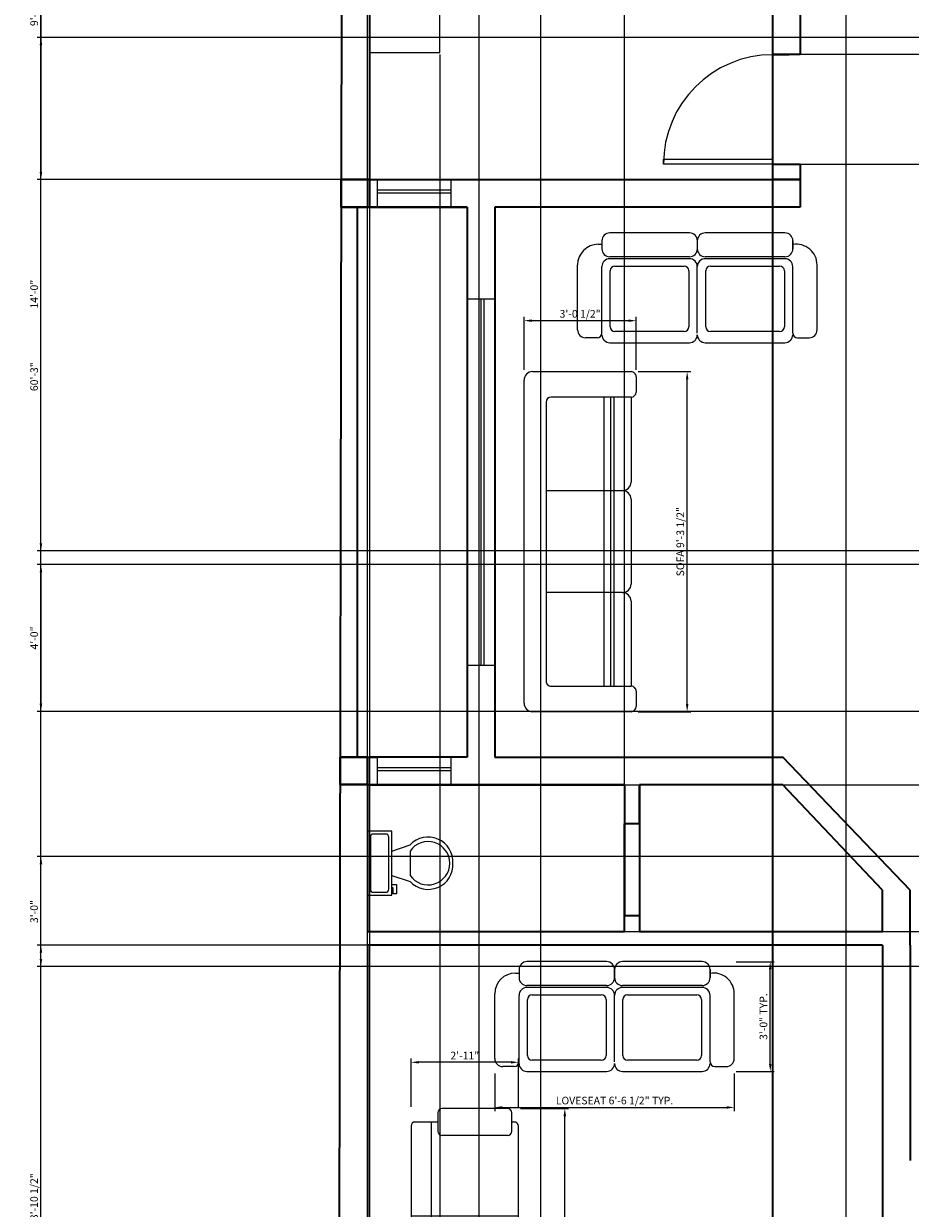
# Model space of a CAD drawing. Units: inches. Extents: x 1624 to 3956, y 1589 to 5028.
# Tile 2 of 16: x 1624 to 1915, y 1862 to 2250. Entities that reach past the tile are written whole.
import ezdxf

# ---------------------------------------------------------------- set-up
doc = ezdxf.new("R2010")
doc.units = ezdxf.units.IN
for name, color, linetype, lineweight in [('A-ANNO-DIMS', 2, 'Continuous', 13), ('A-COLS', 1, 'Continuous', 40), ('A-DOOR', 3, 'Continuous', 18), ('A-FLOR-CASE', 32, 'Continuous', 25), ('A-FLOR-FIXT', 9, 'Continuous', 18), ('A-FURN', 8, 'Continuous', 18), ('A-GLAZ', 4, 'Continuous', 18), ('A-WALL', 7, 'Continuous', 35)]:
    doc.layers.add(name, color=color, linetype=linetype, lineweight=lineweight)
doc.styles.get("Standard").update_dxf_attribs({"font": 'arial.ttf'})
doc.dimstyles.new('Copy of ISO-25', dxfattribs={"dimtxt": 2.5, "dimasz": 2.5, "dimexe": 1.25, "dimexo": 0.625, "dimtad": 1, "dimdec": 1, "dimlunit": 4, "dimtxsty": 'Standard', "dimcen": 2.5, "dimadec": 0, "dimazin": 0, "dimtfac": 1, "dimtdec": 1, "dimtmove": 0, "dimatfit": 3, "dimfxl": 1, "dimarcsym": 0})

# ---------------------------------------------------------------- blocks, each defined once
blk = doc.blocks.new('*U6')
for p, q in [((0, 0), (0, -6)), ((40, 0), (40, -6))]:
    blk.add_line(p, q)
blk.add_lwpolyline([(0, 0), (0, 40), (1.75, 40), (1.75, 0)], close=True)
blk.add_arc((0, 0), 40, 0, 90)
blk = doc.blocks.new('A$C05BA3A2B')
for p, q in [((0.05, 0.6596), (1.95, 0.6596)), ((0.05, 0.6596), (1.95, 0.6596)), ((0.05, 0.6596), (1.95, 0.6596)), ((0, 0.03), (0, 0.6096)), ((0, 0.03), (0, 0.6096)), ((0, 0.03), (0, 0.6096)), ((2, 0.6096), (2, 0.03)), ((2, 0.6096), (2, 0.03)), ((2, 0.6096), (2, 0.03)), ((0.15, 0.5), (0.15, 0.03)), ((0.15, 0.5), (0.15, 0.03)), ((0.15, 0.5), (0.15, 0.03)), ((1.82, 0.53), (0.18, 0.53)), ((1.82, 0.53), (0.18, 0.53)), ((1.82, 0.53), (0.18, 0.53)), ((0.7, 0.08), (0.7, 0.53)), ((0.7, 0.08), (0.7, 0.53)), ((0.7, 0.08), (0.7, 0.53)), ((1.3, 0.53), (1.3, 0.08)), ((1.3, 0.53), (1.3, 0.08)), ((1.3, 0.53), (1.3, 0.08)), ((1.85, 0.03), (1.85, 0.5)), ((1.85, 0.03), (1.85, 0.5)), ((1.85, 0.03), (1.85, 0.5)), ((1.85, 0.1908), (0.15, 0.1908)), ((1.85, 0.1908), (0.15, 0.1908)), ((1.85, 0.1908), (0.15, 0.1908)), ((1.85, 0.1508), (0.15, 0.1508)), ((1.85, 0.1508), (0.15, 0.1508)), ((1.85, 0.1508), (0.15, 0.1508)), ((1.85, 0.1308), (0.15, 0.1308)), ((1.85, 0.1308), (0.15, 0.1308)), ((1.85, 0.1308), (0.15, 0.1308)), ((0.12, 0), (0.03, 0)), ((0.12, 0), (0.03, 0)), ((0.12, 0), (0.03, 0)), ((0.65, 0.03), (0.15, 0.03)), ((0.65, 0.03), (0.15, 0.03)), ((0.65, 0.03), (0.15, 0.03)), ((1.25, 0.03), (0.75, 0.03)), ((1.25, 0.03), (0.75, 0.03)), ((1.25, 0.03), (0.75, 0.03)), ((1.85, 0.03), (1.35, 0.03)), ((1.85, 0.03), (1.35, 0.03)), ((1.85, 0.03), (1.35, 0.03)), ((1.97, 0), (1.88, 0)), ((1.97, 0), (1.88, 0)), ((1.97, 0), (1.88, 0))]:
    blk.add_line(p, q)
for centre, radius, start, end in [((0.05, 0.6096), 0.05, 90, 180), ((0.05, 0.6096), 0.05, 90, 180), ((0.05, 0.6096), 0.05, 90, 180), ((1.95, 0.6096), 0.05, 0, 90), ((1.95, 0.6096), 0.05, 0, 90), ((1.95, 0.6096), 0.05, 0, 90), ((0.18, 0.5), 0.03, 90, 180), ((0.18, 0.5), 0.03, 90, 180), ((0.18, 0.5), 0.03, 90, 180), ((1.82, 0.5), 0.03, 0, 90), ((1.82, 0.5), 0.03, 0, 90), ((1.82, 0.5), 0.03, 0, 90), ((0.65, 0.08), 0.05, 270, 0), ((0.65, 0.08), 0.05, 270, 0), ((0.65, 0.08), 0.05, 270, 0), ((0.75, 0.08), 0.05, 180, 270), ((0.75, 0.08), 0.05, 180, 270), ((0.75, 0.08), 0.05, 180, 270), ((1.25, 0.08), 0.05, 270, 0), ((1.25, 0.08), 0.05, 270, 0), ((1.25, 0.08), 0.05, 270, 0), ((1.35, 0.08), 0.05, 180, 270), ((1.35, 0.08), 0.05, 180, 270), ((1.35, 0.08), 0.05, 180, 270), ((0.03, 0.03), 0.03, 180, 270), ((0.03, 0.03), 0.03, 180, 270), ((0.03, 0.03), 0.03, 180, 270), ((0.12, 0.03), 0.03, 270, 0), ((0.12, 0.03), 0.03, 270, 0), ((0.12, 0.03), 0.03, 270, 0), ((1.88, 0.03), 0.03, 180, 270), ((1.88, 0.03), 0.03, 180, 270), ((1.88, 0.03), 0.03, 180, 270), ((1.97, 0.03), 0.03, 270, 0), ((1.97, 0.03), 0.03, 270, 0), ((1.97, 0.03), 0.03, 270, 0)]:
    blk.add_arc(centre, radius, start, end)
blk = doc.blocks.new('*U14')
for p, q in [((241.3, -152.4), (241.3, -50.8)), ((-254, -215.9), (-203.2, -215.9)), ((-254, -241.3), (-254, -215.9)), ((-177.8, -241.3), (-254, -241.3)), ((-203.2, -215.9), (-203.2, -203.2)), ((-177.8, -203.2), (-177.8, -241.3)), ((-101.6, -203.2), (-152.4, -355.6)), ((101.6, -203.2), (152.4, -355.6)), ((101.6, -355.6), (-101.6, -355.6))]:
    blk.add_line(p, q)
blk.add_lwpolyline([(266.7, -203.2), (266.7, 0), (-266.7, 0), (-266.7, -203.2)], close=True)
for points in [[(-241.3, -50.8), (-241.3, -152.4)], [(215.9, -25.4), (-215.9, -25.4)], [(-215.9, -177.8), (215.9, -177.8)]]:
    blk.add_lwpolyline(points)
for centre, radius, start, end in [((-219.075, -47.625), 22.45064, 81.8699, 188.1301), ((219.075, -47.625), 22.45064, 351.8699, 98.1301), ((-219.075, -155.575), 22.45064, 171.869898, 278.1301), ((219.075, -155.575), 22.45064, 261.8699, 8.1301), ((-12.12088, -505.93752), 205.61935, 133.01722, 273.38), ((0.94996, -504.77674), 181.02486, 124.50543, 269.7), ((-0.94742, -504.77674), 181.02486, 270.3, 55.4946), ((12.12342, -505.93752), 205.61935, 266.62, 46.9828)]:
    blk.add_arc(centre, radius, start, end)
blk = doc.blocks.new('A$C555E41E5')
for p, q in [((0.13, 0.8), (0.8, 0.8)), ((0.8, 0.8), (0.8, 0)), ((0.8, 0.8), (0.8, 0)), ((1.5, 0.8), (0.8, 0.8)), ((2.17, 0.8), (1.5, 0.8)), ((1.5, 0.8), (1.5, 0)), ((1.5, 0.8), (1.5, 0)), ((0.1, 0.6), (0.1, 0.77)), ((2.2, 0.6), (2.2, 0.77)), ((0.1, 0.65), (0.8, 0.65)), ((1.53, 0.65), (0.8, 0.65)), ((2.2, 0.65), (1.5, 0.65)), ((0, 0.08), (0, 0.57)), ((0.03, 0.6), (0.17, 0.6)), ((0.2, 0.08), (0.2, 0.57)), ((2.1, 0.08), (2.1, 0.57)), ((2.27, 0.6), (2.13, 0.6)), ((2.3, 0.08), (2.3, 0.57)), ((0.17, 0.05), (0.03, 0.05)), ((0.1, 0.03), (0.1, 0.05)), ((0.8, 0), (0.13, 0)), ((0.8, 0), (1.5, 0)), ((1.5, 0), (2.17, 0)), ((2.13, 0.05), (2.27, 0.05)), ((2.2, 0.03), (2.2, 0.05))]:
    blk.add_line(p, q)
for centre, start, end in [((0.13, 0.77), 90, 180), ((2.17, 0.77), 0, 90), ((0.03, 0.57), 90, 180), ((0.17, 0.57), 0, 90), ((2.13, 0.57), 90, 180), ((2.27, 0.57), 0, 90), ((0.03, 0.08), 180, 270), ((0.13, 0.03), 180, 270), ((0.17, 0.08), 270, 0), ((2.13, 0.08), 180, 270), ((2.17, 0.03), 270, 0), ((2.27, 0.08), 270, 0)]:
    blk.add_arc(centre, 0.03, start, end)
blk = doc.blocks.new('A$C2BCD7A6E')
blk.add_blockref('A$C555E41E5', (0, 0))
blk = doc.blocks.new('A$C243830B6')
for p, q in [((0.7024, 0.6896), (0.2024, 0.6896)), ((1.3021, 0.6896), (0.8021, 0.6896)), ((0.13, 0.618), (0.15, 0.618)), ((0.1524, 0.6396), (0.1524, 0.5896)), ((0.7521, 0.6396), (0.7521, 0.5896)), ((0.7524, 0.5896), (0.7524, 0.6396)), ((1.3521, 0.6396), (1.3521, 0.5896)), ((1.3524, 0.5896), (1.3524, 0.6396)), ((0.7024, 0.5396), (0.2024, 0.5396)), ((0.7021, 0.5276), (0.2024, 0.5276)), ((1.3021, 0.5396), (0.8021, 0.5396)), ((1.3018, 0.5276), (0.8021, 0.5276)), ((0, 0.0808), (0, 0.488)), ((0.1524, 0.0608), (0.1524, 0.4776)), ((0.2048, 0.1005), (0.2048, 0.4515)), ((0.2348, 0.4815), (0.6691, 0.4815)), ((0.6991, 0.4515), (0.6991, 0.1005)), ((0.7521, 0.0608), (0.7521, 0.4776)), ((0.7521, 0.0608), (0.7521, 0.4776)), ((0.8045, 0.1005), (0.8045, 0.4515)), ((0.8345, 0.4815), (1.2688, 0.4815)), ((1.2988, 0.4515), (1.2988, 0.1005)), ((1.3518, 0.0608), (1.3518, 0.4776)), ((1.3521, 0.0608), (1.3521, 0.4776)), ((1.3521, 0.0608), (1.3521, 0.4776)), ((1.5043, 0.0808), (1.5043, 0.488)), ((0.1224, 0.0308), (0.05, 0.0308)), ((0.2024, 0), (0.7021, 0)), ((0.6691, 0.0705), (0.2348, 0.0705)), ((0.8021, 0), (1.3018, 0)), ((1.2688, 0.0705), (0.8345, 0.0705)), ((1.382, 0.0308), (1.4543, 0.0308))]:
    blk.add_line(p, q)
for centre, radius, start, end in [((0.2024, 0.6396), 0.05, 90, 180), ((0.7024, 0.6396), 0.05, 0, 90), ((0.8021, 0.6396), 0.05, 90, 180), ((1.3021, 0.6396), 0.05, 0, 90), ((0.13, 0.488), 0.13, 90, 180), ((1.3743, 0.488), 0.13, 0, 99.86144), ((0.2024, 0.5896), 0.05, 180, 270), ((0.2024, 0.4776), 0.05, 90, 180), ((0.7021, 0.4776), 0.05, 0, 90), ((0.7024, 0.5896), 0.05, 270, 0), ((0.8021, 0.5896), 0.05, 180, 270), ((0.8021, 0.4776), 0.05, 90, 180), ((1.3018, 0.4776), 0.05, 0, 90), ((1.3021, 0.5896), 0.05, 270, 0), ((0.2348, 0.4515), 0.03, 90, 180), ((0.6691, 0.4515), 0.03, 0, 90), ((0.8345, 0.4515), 0.03, 90, 180), ((1.2688, 0.4515), 0.03, 0, 90), ((0.05, 0.0808), 0.05, 180, 270), ((0.2348, 0.1005), 0.03, 180, 270), ((0.6691, 0.1005), 0.03, 270, 0), ((0.8345, 0.1005), 0.03, 180, 270), ((1.2688, 0.1005), 0.03, 270, 0), ((1.4543, 0.0808), 0.05, 270, 0), ((0.1224, 0.0608), 0.03, 270, 0), ((0.2024, 0.05), 0.05, 180, 270), ((0.7021, 0.05), 0.05, 270, 0), ((0.8021, 0.05), 0.05, 180, 270), ((1.3018, 0.05), 0.05, 270, 0), ((1.382, 0.0608), 0.03, 180, 270)]:
    blk.add_arc(centre, radius, start, end)
blk = doc.blocks.new('WINDOW-24IN')
for p, q in [((0, 0), (0, 9)), ((24, 9), (24, 0)), ((24, 5.5), (0, 5.5)), ((24, 4.5), (0, 4.5))]:
    blk.add_line(p, q)
blk = doc.blocks.new('*D56')
at = {"layer": 'A-ANNO-DIMS', "color": 0, "lineweight": -2, "transparency": 16777216}
for p, q in [((1778.6, 1906.33), (1778.6, 1893.95)), ((1856.98, 1906.33), (1856.98, 1893.95)), ((1781.1, 1895.2), (1854.48, 1895.2))]:
    blk.add_line(p, q, dxfattribs=at)
at = {"layer": 'A-ANNO-DIMS', "color": 0, "transparency": 16777216}
for points in [[(1781.1, 1895.61), (1781.1, 1894.78), (1778.6, 1895.2)], [(1854.48, 1895.61), (1854.48, 1894.78), (1856.98, 1895.2)]]:
    blk.add_solid(points, dxfattribs=at)
at = {"layer": 'Defpoints', "color": 0, "transparency": 16777216}
for p in [(1778.6, 1906.96), (1856.98, 1906.96), (1856.98, 1895.2)]:
    blk.add_point(p, dxfattribs=at)
at = {"layer": 'A-ANNO-DIMS', "color": 0, "transparency": 16777216, "insert": (1817.79, 1897.12), "char_height": 2.5, "attachment_point": 5}
blk.add_mtext('LOVESEAT 6\'-6 1/2" TYP.', dxfattribs=at)
blk = doc.blocks.new('*D57')
at = {"layer": 'A-ANNO-DIMS', "color": 0, "lineweight": -2, "transparency": 16777216}
for p, q in [((1857.61, 1942.89), (1869.99, 1942.89)), ((1868.74, 1909.46), (1868.74, 1940.39)), ((1857.61, 1906.96), (1869.99, 1906.96))]:
    blk.add_line(p, q, dxfattribs=at)
at = {"layer": 'A-ANNO-DIMS', "color": 0, "transparency": 16777216}
for points in [[(1868.32, 1940.39), (1869.16, 1940.39), (1868.74, 1942.89)], [(1868.32, 1909.46), (1869.16, 1909.46), (1868.74, 1906.96)]]:
    blk.add_solid(points, dxfattribs=at)
at = {"layer": 'Defpoints', "color": 0, "transparency": 16777216}
for p in [(1856.98, 1942.89), (1868.74, 1942.89), (1856.98, 1906.96)]:
    blk.add_point(p, dxfattribs=at)
at = {"layer": 'A-ANNO-DIMS', "color": 0, "transparency": 16777216, "insert": (1866.84, 1924.92), "char_height": 2.5, "attachment_point": 5, "rotation": 90}
blk.add_mtext('3\'-0" TYP.', dxfattribs=at)
blk = doc.blocks.new('*D62')
at = {"layer": 'A-ANNO-DIMS', "color": 0, "lineweight": -2, "transparency": 16777216}
for p, q in [((1825.5, 2135.94), (1842.81, 2135.94)), ((1841.56, 2027.19), (1841.56, 2133.44)), ((1825.5, 2024.69), (1842.81, 2024.69))]:
    blk.add_line(p, q, dxfattribs=at)
at = {"layer": 'A-ANNO-DIMS', "color": 0, "transparency": 16777216}
for points in [[(1841.14, 2133.44), (1841.98, 2133.44), (1841.56, 2135.94)], [(1841.14, 2027.19), (1841.98, 2027.19), (1841.56, 2024.69)]]:
    blk.add_solid(points, dxfattribs=at)
at = {"layer": 'Defpoints', "color": 0, "transparency": 16777216}
for p in [(1824.87, 2135.94), (1841.56, 2135.94), (1824.87, 2024.69)]:
    blk.add_point(p, dxfattribs=at)
at = {"layer": 'A-ANNO-DIMS', "color": 0, "transparency": 16777216, "insert": (1839.64, 2080.31), "char_height": 2.5, "attachment_point": 5, "rotation": 90}
blk.add_mtext('SOFA 9\'-3 1/2"', dxfattribs=at)
blk = doc.blocks.new('*D63')
at = {"layer": 'A-ANNO-DIMS', "color": 0, "lineweight": -2, "transparency": 16777216}
for p, q in [((1788.18, 2136.56), (1788.18, 2153.87)), ((1822.37, 2152.62), (1790.68, 2152.62)), ((1824.87, 2136.56), (1824.87, 2153.87))]:
    blk.add_line(p, q, dxfattribs=at)
at = {"layer": 'A-ANNO-DIMS', "color": 0, "transparency": 16777216}
for points in [[(1790.68, 2153.04), (1790.68, 2152.21), (1788.18, 2152.62)], [(1822.37, 2153.04), (1822.37, 2152.21), (1824.87, 2152.62)]]:
    blk.add_solid(points, dxfattribs=at)
at = {"layer": 'Defpoints', "color": 0, "transparency": 16777216}
for p in [(1788.18, 2152.62), (1788.18, 2135.94), (1824.87, 2135.94)]:
    blk.add_point(p, dxfattribs=at)
at = {"layer": 'A-ANNO-DIMS', "color": 0, "transparency": 16777216, "insert": (1806.53, 2154.54), "char_height": 2.5, "attachment_point": 5}
blk.add_mtext('3\'-0 1/2"', dxfattribs=at)
blk = doc.blocks.new('*D64')
at = {"layer": 'A-ANNO-DIMS', "color": 0, "lineweight": -2, "transparency": 16777216}
for p, q in [((1787, 1894.81), (1802.77, 1894.81)), ((1801.52, 1796.3), (1801.52, 1892.31)), ((1787, 1793.8), (1802.77, 1793.8))]:
    blk.add_line(p, q, dxfattribs=at)
at = {"layer": 'A-ANNO-DIMS', "color": 0, "transparency": 16777216}
for points in [[(1801.11, 1892.31), (1801.94, 1892.31), (1801.52, 1894.81)], [(1801.11, 1796.3), (1801.94, 1796.3), (1801.52, 1793.8)]]:
    blk.add_solid(points, dxfattribs=at)
at = {"layer": 'Defpoints', "color": 0, "transparency": 16777216}
for p in [(1786.37, 1894.81), (1801.52, 1894.81), (1786.37, 1793.8)]:
    blk.add_point(p, dxfattribs=at)
at = {"layer": 'A-ANNO-DIMS', "color": 0, "transparency": 16777216, "insert": (1799.6, 1844.31), "char_height": 2.5, "attachment_point": 5, "rotation": 90}
blk.add_mtext('SOFA 8\'-5"', dxfattribs=at)
blk = doc.blocks.new('*D65')
at = {"layer": 'A-ANNO-DIMS', "color": 0, "lineweight": -2, "transparency": 16777216}
for p, q in [((1751.23, 1895.44), (1751.23, 1911.22)), ((1786.37, 1895.44), (1786.37, 1911.22)), ((1783.87, 1909.97), (1753.73, 1909.97))]:
    blk.add_line(p, q, dxfattribs=at)
at = {"layer": 'A-ANNO-DIMS', "color": 0, "transparency": 16777216}
for points in [[(1753.73, 1910.38), (1753.73, 1909.55), (1751.23, 1909.97)], [(1783.87, 1910.38), (1783.87, 1909.55), (1786.37, 1909.97)]]:
    blk.add_solid(points, dxfattribs=at)
at = {"layer": 'Defpoints', "color": 0, "transparency": 16777216}
for p in [(1751.23, 1909.97), (1751.23, 1894.81), (1786.37, 1894.81)]:
    blk.add_point(p, dxfattribs=at)
at = {"layer": 'A-ANNO-DIMS', "color": 0, "transparency": 16777216, "insert": (1768.8, 1911.85), "char_height": 2.5, "attachment_point": 5}
blk.add_mtext('2\'-11"', dxfattribs=at)
blk = doc.blocks.new('*D69')
at = {"layer": 'A-ANNO-DIMS', "color": 0, "lineweight": -2, "transparency": 16777216}
for p, q in [((1727.95, 2495.79), (1628.86, 2495.79)), ((1630.11, 1775.29), (1630.11, 2493.29)), ((1726.95, 1772.79), (1628.86, 1772.79))]:
    blk.add_line(p, q, dxfattribs=at)
at = {"layer": 'A-ANNO-DIMS', "color": 0, "transparency": 16777216}
for points in [[(1629.69, 2493.29), (1630.53, 2493.29), (1630.11, 2495.79)], [(1629.69, 1775.29), (1630.53, 1775.29), (1630.11, 1772.79)]]:
    blk.add_solid(points, dxfattribs=at)
at = {"layer": 'Defpoints', "color": 0, "transparency": 16777216}
for p in [(1630.11, 2495.79), (1728.58, 2495.79), (1727.58, 1772.79)]:
    blk.add_point(p, dxfattribs=at)
at = {"layer": 'A-ANNO-DIMS', "color": 0, "transparency": 16777216, "insert": (1628.21, 2134.29), "char_height": 2.5, "attachment_point": 5, "rotation": 90}
blk.add_mtext('60\'-3"', dxfattribs=at)
blk = doc.blocks.new('*D75')
at = {"layer": 'A-ANNO-DIMS', "color": 0, "lineweight": -2, "transparency": 16777216}
for p, q in [((1737.58, 2486.17), (1737.58, 1589.9)), ((1793.58, 2486.17), (1793.58, 1589.9)), ((1740.08, 1591.15), (1791.08, 1591.15))]:
    blk.add_line(p, q, dxfattribs=at)
at = {"layer": 'A-ANNO-DIMS', "color": 0, "transparency": 16777216}
for points in [[(1740.08, 1591.57), (1740.08, 1590.73), (1737.58, 1591.15)], [(1791.08, 1591.57), (1791.08, 1590.73), (1793.58, 1591.15)]]:
    blk.add_solid(points, dxfattribs=at)
at = {"layer": 'Defpoints', "color": 0, "transparency": 16777216}
for p in [(1737.58, 2486.79), (1793.58, 2486.79), (1793.58, 1591.15)]:
    blk.add_point(p, dxfattribs=at)
at = {"layer": 'A-ANNO-DIMS', "color": 0, "transparency": 16777216, "insert": (1765.58, 1593.05), "char_height": 2.5, "attachment_point": 5}
blk.add_mtext('4\'-8"', dxfattribs=at)
blk = doc.blocks.new('*D82')
at = {"layer": 'A-ANNO-DIMS', "color": 0, "lineweight": -2, "transparency": 16777216}
for p, q in [((1737.58, 2306.17), (1737.58, 1589.9)), ((1869.56, 2306.17), (1869.56, 1589.9)), ((1740.08, 1591.15), (1867.06, 1591.15))]:
    blk.add_line(p, q, dxfattribs=at)
at = {"layer": 'A-ANNO-DIMS', "color": 0, "transparency": 16777216}
for points in [[(1740.08, 1591.57), (1740.08, 1590.73), (1737.58, 1591.15)], [(1867.06, 1591.57), (1867.06, 1590.73), (1869.56, 1591.15)]]:
    blk.add_solid(points, dxfattribs=at)
at = {"layer": 'Defpoints', "color": 0, "transparency": 16777216}
for p in [(1737.58, 2306.79), (1869.56, 2306.79), (1869.56, 1591.15)]:
    blk.add_point(p, dxfattribs=at)
at = {"layer": 'A-ANNO-DIMS', "color": 0, "transparency": 16777216, "insert": (1803.57, 1593.05), "char_height": 2.5, "attachment_point": 5}
blk.add_mtext('11\'-0"', dxfattribs=at)
blk = doc.blocks.new('*D83')
at = {"layer": 'A-ANNO-DIMS', "color": 0, "lineweight": -2, "transparency": 16777216}
for p, q in [((1868.93, 2306.79), (1628.86, 2306.79)), ((1630.11, 2304.29), (1630.11, 2201.29)), ((1868.93, 2198.79), (1628.86, 2198.79))]:
    blk.add_line(p, q, dxfattribs=at)
at = {"layer": 'A-ANNO-DIMS', "color": 0, "transparency": 16777216}
for points in [[(1629.69, 2304.29), (1630.53, 2304.29), (1630.11, 2306.79)], [(1629.69, 2201.29), (1630.53, 2201.29), (1630.11, 2198.79)]]:
    blk.add_solid(points, dxfattribs=at)
at = {"layer": 'Defpoints', "color": 0, "transparency": 16777216}
for p in [(1869.56, 2306.79), (1630.11, 2198.79), (1869.56, 2198.79)]:
    blk.add_point(p, dxfattribs=at)
at = {"layer": 'A-ANNO-DIMS', "color": 0, "transparency": 16777216, "insert": (1628.21, 2252.79), "char_height": 2.5, "attachment_point": 5, "rotation": 90}
blk.add_mtext('9\'-0"', dxfattribs=at)
blk = doc.blocks.new('*D84')
at = {"layer": 'A-ANNO-DIMS', "color": 0, "lineweight": -2, "transparency": 16777216}
for p, q in [((1904.9, 1948.29), (1628.86, 1948.29)), ((1630.11, 1784.29), (1630.11, 1945.79)), ((1904.9, 1781.79), (1628.86, 1781.79))]:
    blk.add_line(p, q, dxfattribs=at)
at = {"layer": 'A-ANNO-DIMS', "color": 0, "transparency": 16777216}
for points in [[(1629.69, 1945.79), (1630.53, 1945.79), (1630.11, 1948.29)], [(1629.69, 1784.29), (1630.53, 1784.29), (1630.11, 1781.79)]]:
    blk.add_solid(points, dxfattribs=at)
at = {"layer": 'Defpoints', "color": 0, "transparency": 16777216}
for p in [(1630.11, 1948.29), (1905.53, 1948.29), (1905.53, 1781.79)]:
    blk.add_point(p, dxfattribs=at)
at = {"layer": 'A-ANNO-DIMS', "color": 0, "transparency": 16777216, "insert": (1628.19, 1865.04), "char_height": 2.5, "attachment_point": 5, "rotation": 90}
blk.add_mtext('13\'-10 1/2"', dxfattribs=at)
blk = doc.blocks.new('*D86')
at = {"layer": 'A-ANNO-DIMS', "color": 0, "lineweight": -2, "transparency": 16777216}
for p, q in [((1737.01, 1953.42), (1737.01, 2612.84)), ((1821.01, 1953.42), (1821.01, 2612.84)), ((1739.51, 2611.59), (1818.51, 2611.59))]:
    blk.add_line(p, q, dxfattribs=at)
at = {"layer": 'A-ANNO-DIMS', "color": 0, "transparency": 16777216}
for points in [[(1739.51, 2612.01), (1739.51, 2611.18), (1737.01, 2611.59)], [(1818.51, 2612.01), (1818.51, 2611.18), (1821.01, 2611.59)]]:
    blk.add_solid(points, dxfattribs=at)
at = {"layer": 'Defpoints', "color": 0, "transparency": 16777216}
for p in [(1821.01, 2611.59), (1737.01, 1952.79), (1821.01, 1952.79)]:
    blk.add_point(p, dxfattribs=at)
at = {"layer": 'A-ANNO-DIMS', "color": 0, "transparency": 16777216, "insert": (1779.01, 2613.5), "char_height": 2.5, "attachment_point": 5}
blk.add_mtext('7\'-0"', dxfattribs=at)
blk = doc.blocks.new('*D87')
at = {"layer": 'A-ANNO-DIMS', "color": 0, "lineweight": -2, "transparency": 16777216}
for p, q in [((1737.64, 2000.79), (2217.63, 2000.79)), ((2216.38, 1998.29), (2216.38, 1955.29)), ((1737.64, 1952.79), (2217.63, 1952.79))]:
    blk.add_line(p, q, dxfattribs=at)
at = {"layer": 'A-ANNO-DIMS', "color": 0, "transparency": 16777216}
for points in [[(2215.96, 1998.29), (2216.8, 1998.29), (2216.38, 2000.79)], [(2215.96, 1955.29), (2216.8, 1955.29), (2216.38, 1952.79)]]:
    blk.add_solid(points, dxfattribs=at)
at = {"layer": 'Defpoints', "color": 0, "transparency": 16777216}
for p in [(1737.01, 2000.79), (1737.01, 1952.79), (2216.38, 1952.79)]:
    blk.add_point(p, dxfattribs=at)
at = {"layer": 'A-ANNO-DIMS', "color": 0, "transparency": 16777216, "insert": (2214.48, 1976.79), "char_height": 2.5, "attachment_point": 5, "rotation": 90}
blk.add_mtext('4\'-0"', dxfattribs=at)
blk = doc.blocks.new('*D91')
at = {"layer": 'A-ANNO-DIMS', "color": 0, "lineweight": -2, "transparency": 16777216}
for p, q in [((2054.95, 1977.29), (1628.86, 1977.29)), ((1630.11, 1943.79), (1630.11, 1974.79)), ((2054.95, 1941.29), (1628.86, 1941.29))]:
    blk.add_line(p, q, dxfattribs=at)
at = {"layer": 'A-ANNO-DIMS', "color": 0, "transparency": 16777216}
for points in [[(1629.69, 1974.79), (1630.53, 1974.79), (1630.11, 1977.29)], [(1629.69, 1943.79), (1630.53, 1943.79), (1630.11, 1941.29)]]:
    blk.add_solid(points, dxfattribs=at)
at = {"layer": 'Defpoints', "color": 0, "transparency": 16777216}
for p in [(1630.11, 1977.29), (2055.58, 1977.29), (2055.58, 1941.29)]:
    blk.add_point(p, dxfattribs=at)
at = {"layer": 'A-ANNO-DIMS', "color": 0, "transparency": 16777216, "insert": (1628.21, 1959.29), "char_height": 2.5, "attachment_point": 5, "rotation": 90}
blk.add_mtext('3\'-0"', dxfattribs=at)
blk = doc.blocks.new('*D93')
at = {"layer": 'A-ANNO-DIMS', "color": 0, "lineweight": -2, "transparency": 16777216}
for p, q in [((2090.95, 2072.79), (1628.86, 2072.79)), ((1630.11, 2070.29), (1630.11, 2027.29)), ((2090.95, 2024.79), (1628.86, 2024.79))]:
    blk.add_line(p, q, dxfattribs=at)
at = {"layer": 'A-ANNO-DIMS', "color": 0, "transparency": 16777216}
for points in [[(1629.69, 2070.29), (1630.53, 2070.29), (1630.11, 2072.79)], [(1629.69, 2027.29), (1630.53, 2027.29), (1630.11, 2024.79)]]:
    blk.add_solid(points, dxfattribs=at)
at = {"layer": 'Defpoints', "color": 0, "transparency": 16777216}
for p in [(2091.58, 2072.79), (1630.11, 2024.79), (2091.58, 2024.79)]:
    blk.add_point(p, dxfattribs=at)
at = {"layer": 'A-ANNO-DIMS', "color": 0, "transparency": 16777216, "insert": (1628.21, 2048.79), "char_height": 2.5, "attachment_point": 5, "rotation": 90}
blk.add_mtext('4\'-0"', dxfattribs=at)
blk = doc.blocks.new('*D94')
at = {"layer": 'A-ANNO-DIMS', "color": 0, "lineweight": -2, "transparency": 16777216}
for p, q in [((1893.52, 2315.17), (1893.52, 1589.9)), ((1929.52, 2315.17), (1929.52, 1589.9)), ((1896.02, 1591.15), (1927.02, 1591.15))]:
    blk.add_line(p, q, dxfattribs=at)
at = {"layer": 'A-ANNO-DIMS', "color": 0, "transparency": 16777216}
for points in [[(1896.02, 1591.57), (1896.02, 1590.73), (1893.52, 1591.15)], [(1927.02, 1591.57), (1927.02, 1590.73), (1929.52, 1591.15)]]:
    blk.add_solid(points, dxfattribs=at)
at = {"layer": 'Defpoints', "color": 0, "transparency": 16777216}
for p in [(1893.52, 2315.79), (1929.52, 2315.79), (1929.52, 1591.15)]:
    blk.add_point(p, dxfattribs=at)
at = {"layer": 'A-ANNO-DIMS', "color": 0, "transparency": 16777216, "insert": (1911.52, 1593.05), "char_height": 2.5, "attachment_point": 5}
blk.add_mtext('3\'-0"', dxfattribs=at)
blk = doc.blocks.new('*D95')
at = {"layer": 'A-ANNO-DIMS', "color": 0, "lineweight": -2, "transparency": 16777216}
for p, q in [((1870.18, 2239.87), (2217.63, 2239.87)), ((2216.38, 2206.37), (2216.38, 2237.37)), ((1870.18, 2203.87), (2217.63, 2203.87))]:
    blk.add_line(p, q, dxfattribs=at)
at = {"layer": 'A-ANNO-DIMS', "color": 0, "transparency": 16777216}
for points in [[(2215.96, 2237.37), (2216.8, 2237.37), (2216.38, 2239.87)], [(2215.96, 2206.37), (2216.8, 2206.37), (2216.38, 2203.87)]]:
    blk.add_solid(points, dxfattribs=at)
at = {"layer": 'Defpoints', "color": 0, "transparency": 16777216}
for p in [(1869.56, 2239.87), (2216.38, 2239.87), (1869.56, 2203.87)]:
    blk.add_point(p, dxfattribs=at)
at = {"layer": 'A-ANNO-DIMS', "color": 0, "transparency": 16777216, "insert": (2214.48, 2221.87), "char_height": 2.5, "attachment_point": 5, "rotation": 90}
blk.add_mtext('3\'-0"', dxfattribs=at)
blk = doc.blocks.new('*D97')
at = {"layer": 'A-ANNO-DIMS', "color": 0, "lineweight": -2, "transparency": 16777216}
for p, q in [((1773.53, 1773.42), (1773.53, 2612.84)), ((1869.53, 1773.42), (1869.53, 2612.84)), ((1776.03, 2611.59), (1867.03, 2611.59))]:
    blk.add_line(p, q, dxfattribs=at)
at = {"layer": 'A-ANNO-DIMS', "color": 0, "transparency": 16777216}
for points in [[(1776.03, 2612.01), (1776.03, 2611.18), (1773.53, 2611.59)], [(1867.03, 2612.01), (1867.03, 2611.18), (1869.53, 2611.59)]]:
    blk.add_solid(points, dxfattribs=at)
at = {"layer": 'Defpoints', "color": 0, "transparency": 16777216}
for p in [(1869.53, 2611.59), (1773.53, 1772.79), (1869.53, 1772.79)]:
    blk.add_point(p, dxfattribs=at)
at = {"layer": 'A-ANNO-DIMS', "color": 0, "transparency": 16777216, "insert": (1821.53, 2613.5), "char_height": 2.5, "attachment_point": 5}
blk.add_mtext('8\'-0"', dxfattribs=at)
blk = doc.blocks.new('*D98')
at = {"layer": 'A-ANNO-DIMS', "color": 0, "lineweight": -2, "transparency": 16777216}
for p, q in [((2090.95, 2245.29), (1628.86, 2245.29)), ((1630.11, 2079.79), (1630.11, 2242.79)), ((2090.95, 2077.29), (1628.86, 2077.29))]:
    blk.add_line(p, q, dxfattribs=at)
at = {"layer": 'A-ANNO-DIMS', "color": 0, "transparency": 16777216}
for points in [[(1629.69, 2242.79), (1630.53, 2242.79), (1630.11, 2245.29)], [(1629.69, 2079.79), (1630.53, 2079.79), (1630.11, 2077.29)]]:
    blk.add_solid(points, dxfattribs=at)
at = {"layer": 'Defpoints', "color": 0, "transparency": 16777216}
for p in [(1630.11, 2245.29), (2091.58, 2245.29), (2091.58, 2077.29)]:
    blk.add_point(p, dxfattribs=at)
at = {"layer": 'A-ANNO-DIMS', "color": 0, "transparency": 16777216, "insert": (1628.21, 2161.29), "char_height": 2.5, "attachment_point": 5, "rotation": 90}
blk.add_mtext('14\'-0"', dxfattribs=at)
blk = doc.blocks.new('*D99')
at = {"layer": 'A-ANNO-DIMS', "color": 0, "lineweight": -2, "transparency": 16777216}
for p, q in [((1737.58, 2239.75), (1737.58, 1589.9)), ((1760.58, 2239.75), (1760.58, 1589.9)), ((1740.08, 1591.15), (1758.08, 1591.15))]:
    blk.add_line(p, q, dxfattribs=at)
at = {"layer": 'A-ANNO-DIMS', "color": 0, "transparency": 16777216}
for points in [[(1740.08, 1591.57), (1740.08, 1590.73), (1737.58, 1591.15)], [(1758.08, 1591.57), (1758.08, 1590.73), (1760.58, 1591.15)]]:
    blk.add_solid(points, dxfattribs=at)
at = {"layer": 'Defpoints', "color": 0, "transparency": 16777216}
for p in [(1737.58, 2240.37), (1760.58, 2240.37), (1760.58, 1591.15)]:
    blk.add_point(p, dxfattribs=at)
at = {"layer": 'A-ANNO-DIMS', "color": 0, "transparency": 16777216, "insert": (1749.08, 1593.03), "char_height": 2.5, "attachment_point": 5}
blk.add_mtext('1\'-11"', dxfattribs=at)
blk = doc.blocks.new('*D101')
at = {"layer": 'A-ANNO-DIMS', "color": 0, "lineweight": -2, "transparency": 16777216}
for p, q in [((1737.01, 1782.42), (1737.01, 2612.84)), ((1773.53, 1782.42), (1773.53, 2612.84)), ((1739.51, 2611.59), (1771.03, 2611.59))]:
    blk.add_line(p, q, dxfattribs=at)
at = {"layer": 'A-ANNO-DIMS', "color": 0, "transparency": 16777216}
for points in [[(1739.51, 2612.01), (1739.51, 2611.18), (1737.01, 2611.59)], [(1771.03, 2612.01), (1771.03, 2611.18), (1773.53, 2611.59)]]:
    blk.add_solid(points, dxfattribs=at)
at = {"layer": 'Defpoints', "color": 0, "transparency": 16777216}
for p in [(1773.53, 2611.59), (1737.01, 1781.79), (1773.53, 1781.79)]:
    blk.add_point(p, dxfattribs=at)
at = {"layer": 'A-ANNO-DIMS', "color": 0, "transparency": 16777216, "insert": (1755.27, 2613.51), "char_height": 2.5, "attachment_point": 5}
blk.add_mtext('3\'-0 1/2"', dxfattribs=at)

msp = doc.modelspace()

# ---------------------------------------------------------------- linework, layer by layer
at = {"layer": 'A-COLS'}
for p, q in [((1728.37, 2189.81), (1728.38, 2198.81)), ((1737.58, 2198.79), (1728.38, 2198.81)), ((1728.38, 2198.81), (1737.58, 2198.79)), ((1737.58, 2198.79), (1737.58, 2189.79)), ((1737.58, 2189.79), (1728.37, 2189.81)), ((1728.03, 2009.81), (1728.01, 2000.81)), ((1737.01, 2009.79), (1728.03, 2009.81)), ((1737.01, 2000.79), (1737.01, 2009.79)), ((1737.01, 2000.79), (1737.01, 2009.79)), ((1728.01, 2000.81), (1737.01, 2000.81))]:
    msp.add_line(p, q, dxfattribs=at)
at = {"layer": 'A-FLOR-CASE'}
for p, q in [((1760.58, 2240.37), (1760.58, 2283.78)), ((1737.58, 2240.37), (1760.58, 2240.37)), ((1737.58, 2240.37), (1760.58, 2240.37))]:
    msp.add_line(p, q, dxfattribs=at)
at = {"layer": 'A-GLAZ'}
for p, q in [((1740.27, 2198.79), (1764.27, 2198.79)), ((1769.58, 2159.79), (1778.58, 2159.79)), ((1774.08, 2159.79), (1774.08, 2039.79)), ((1775.08, 2159.79), (1775.08, 2039.79)), ((1778.58, 2159.79), (1778.58, 2039.79)), ((1778.58, 2039.79), (1769.58, 2039.79))]:
    msp.add_line(p, q, dxfattribs=at)
at = {"layer": 'A-WALL'}
for p, q in [((1737.58, 2306.79), (1737.58, 2198.79)), ((1869.56, 2239.87), (1869.56, 2306.79)), ((1878.56, 2306.79), (1878.56, 2239.87)), ((1728.58, 2301.8), (1727.58, 1772.79)), ((1869.56, 2239.87), (1878.56, 2239.87)), ((1869.56, 2198.79), (1869.56, 2203.87)), ((1869.56, 2203.87), (1878.56, 2203.87)), ((1878.56, 2203.87), (1878.56, 2198.79)), ((1737.58, 2198.79), (1878.56, 2198.79)), ((1878.56, 2198.79), (1869.56, 2198.79)), ((1878.56, 2198.79), (1878.56, 2189.79)), ((1737.58, 2189.79), (1733.58, 2189.79)), ((1733.58, 2189.79), (1733.58, 2009.79)), ((1737.58, 2189.79), (1769.58, 2189.79)), ((1769.58, 2189.79), (1737.58, 2189.79)), ((1769.58, 2189.79), (1769.58, 2009.79)), ((1769.58, 2189.79), (1769.58, 2159.79)), ((1782.58, 2189.79), (1778.58, 2189.79)), ((1778.58, 2189.79), (1778.58, 2009.79)), ((1878.56, 2189.79), (1782.58, 2189.79)), ((1733.58, 2009.79), (1737.58, 2009.79)), ((1737.01, 2009.79), (1740.27, 2009.79)), ((1769.58, 2009.79), (1737.58, 2009.79)), ((1778.58, 2009.79), (1872.81, 2009.79)), ((1914.53, 1966.3), (1872.81, 2009.79)), ((1872.81, 2009.79), (1872.81, 2009.79)), ((1737.58, 2000.79), (1737.01, 2000.79)), ((1737.01, 2000.79), (1737.01, 1952.79)), ((1737.01, 2000.79), (1821.01, 2000.79)), ((1737.01, 2000.79), (1737.01, 1952.79)), ((1737.01, 2000.79), (1737.01, 2000.79)), ((1773.58, 2000.79), (1737.58, 2000.79)), ((1740.27, 2000.79), (1755.58, 2000.79)), ((1778.58, 2000.79), (1773.58, 2000.79)), ((1821.01, 2000.79), (1778.58, 2000.79)), ((1821.01, 2000.79), (1821.01, 1988.04)), ((1872.81, 2000.79), (1826.01, 2000.79)), ((1826.01, 1988.04), (1826.01, 2000.79)), ((1826.01, 2000.79), (1826.01, 1988.04)), ((1905.53, 1966.3), (1872.81, 2000.79)), ((1821.01, 1952.79), (1821.01, 1988.04)), ((1826.01, 1988.04), (1821.01, 1988.04)), ((1821.01, 1988.04), (1821.01, 1958.04)), ((1826.01, 1988.04), (1826.01, 1952.79)), ((1905.53, 1952.79), (1905.53, 1966.3)), ((1914.53, 1948.29), (1914.53, 1966.3)), ((1821.01, 1958.04), (1826.01, 1958.04)), ((1737.01, 1952.79), (1821.01, 1952.79)), ((1826.01, 1952.79), (1905.53, 1952.79)), ((1826.01, 1948.29), (1737.01, 1948.29)), ((1737.01, 1948.29), (1737.01, 1781.79)), ((1905.53, 1948.29), (1826.01, 1948.29)), ((1905.53, 1948.29), (1905.53, 1781.79)), ((1914.53, 1948.29), (1914.57, 1877.79)), ((1914.58, 1877.79), (1914.57, 1877.79))]:
    msp.add_line(p, q, dxfattribs=at)

# ---------------------------------------------------------------- block references
at = {"layer": 'A-DOOR', "xscale": 0.8941036658146853, "yscale": 0.8941036658146853, "zscale": 0.8941036658146853, "rotation": 89.99999999999999}
msp.add_blockref('*U6', (1869.56, 2203.87), dxfattribs=at)
at = {"layer": 'A-FLOR-FIXT', "xscale": 0.0393700787401575, "yscale": 0.0393700787401575, "zscale": 0.0393700787401575, "rotation": 89.99999999999999}
msp.add_blockref('*U14', (1736.91, 1975.1), dxfattribs=at)
at = {"layer": 'A-FURN', "xscale": 52.10375933184375, "yscale": 52.10375933184375, "zscale": 52.10375933184375}
for p in [(1805.7, 2145.42), (1778.6, 1906.96)]:
    msp.add_blockref('A$C243830B6', p, dxfattribs=at)
at = {"layer": 'A-FURN'}
for name, p, xscale, yscale, zscale, rotation in [('A$C05BA3A2B', (1824.87, 2024.69), 55.62516327614314, 55.62516327614314, 55.62516327614314, 89.99999999999999), ('A$C2BCD7A6E', (1786.37, 1793.8), 43.92080760397013, 43.92080760397013, 43.92080760397013, 90)]:
    msp.add_blockref(name, p, dxfattribs=dict(at, xscale=xscale, yscale=yscale, zscale=zscale, rotation=rotation))
at = {"layer": 'A-GLAZ'}
for p in [(1740.27, 2189.79), (1740.27, 2000.79)]:
    msp.add_blockref('WINDOW-24IN', p, dxfattribs=at)

# ---------------------------------------------------------------- dimensions: what is measured, and where the dimension line sits
at = {"layer": 'A-ANNO-DIMS'}
for base, p1, p2, picture, middle in [((1773.53, 2611.59), (1737.01, 1781.79), (1773.53, 1781.79), '*D101', (1755.27, 2613.51)), ((1821.01, 2611.59), (1737.01, 1952.79), (1821.01, 1952.79), '*D86', (1779.01, 2613.5)), ((1869.53, 2611.59), (1773.53, 1772.79), (1869.53, 1772.79), '*D97', (1821.53, 2613.5)), ((1793.58, 1591.15), (1737.58, 2486.79), (1793.58, 2486.79), '*D75', (1765.58, 1593.05)), ((1929.52, 1591.15), (1893.52, 2315.79), (1929.52, 2315.79), '*D94', (1911.52, 1593.05)), ((1869.56, 1591.15), (1737.58, 2306.79), (1869.56, 2306.79), '*D82', (1803.57, 1593.05)), ((1760.58, 1591.15), (1737.58, 2240.37), (1760.58, 2240.37), '*D99', (1749.08, 1593.03))]:
    dim = msp.add_linear_dim(base=base, p1=p1, p2=p2, dimstyle='Copy of ISO-25', override={"dimdec": 1, "dimlfac": 1, "dimrnd": 0, "dimzin": 1, "dimdsep": 46, "dimlunit": 4, "dimfrac": 2}, dxfattribs=at)
    dim.commit()
    dim.dimension.update_dxf_attribs({"geometry": picture, "text_midpoint": middle})
for base, p1, p2, angle, picture, middle in [((1630.11, 2495.79), (1727.58, 1772.79), (1728.58, 2495.79), 90, '*D69', (1628.21, 2134.29)), ((1630.11, 2198.79), (1869.56, 2306.79), (1869.56, 2198.79), 90, '*D83', (1628.21, 2252.79)), ((1630.11, 2245.29), (2091.58, 2077.29), (2091.58, 2245.29), 90, '*D98', (1628.21, 2161.29)), ((2216.38, 2239.87), (1869.56, 2203.87), (1869.56, 2239.87), 90, '*D95', (2214.48, 2221.87)), ((1788.18, 2152.62), (1824.87, 2135.94), (1788.18, 2135.94), 180, '*D63', (1806.53, 2154.54)), ((1630.11, 2024.79), (2091.58, 2072.79), (2091.58, 2024.79), 90, '*D93', (1628.21, 2048.79)), ((2216.38, 1952.79), (1737.01, 2000.79), (1737.01, 1952.79), 90, '*D87', (2214.48, 1976.79)), ((1630.11, 1977.29), (2055.58, 1941.29), (2055.58, 1977.29), 90, '*D91', (1628.21, 1959.29)), ((1630.11, 1948.29), (1905.53, 1781.79), (1905.53, 1948.29), 90, '*D84', (1628.19, 1865.04)), ((1751.23, 1909.97), (1786.37, 1894.81), (1751.23, 1894.81), 180, '*D65', (1768.8, 1911.85))]:
    dim = msp.add_linear_dim(base=base, p1=p1, p2=p2, angle=angle, dimstyle='Copy of ISO-25', override={"dimdec": 1, "dimlfac": 1, "dimrnd": 0, "dimzin": 1, "dimdsep": 46, "dimlunit": 4, "dimfrac": 2}, dxfattribs=at)
    dim.commit()
    dim.dimension.update_dxf_attribs({"geometry": picture, "text_midpoint": middle})
for base, p1, p2, text, picture, middle in [((1841.5592, 2135.9365), (1824.8717, 2024.6861), (1824.8717, 2135.9365), 'SOFA <>', '*D62', (1839.6399, 2080.3113)), ((1868.74, 1942.89), (1856.98, 1906.96), (1856.98, 1942.89), '<> TYP.', '*D57', (1866.84, 1924.92)), ((1801.52, 1894.81), (1786.37, 1793.8), (1786.37, 1894.81), 'SOFA <>', '*D64', (1799.6, 1844.31))]:
    dim = msp.add_linear_dim(base=base, p1=p1, p2=p2, angle=90, text=text, dimstyle='Copy of ISO-25', override={"dimdec": 1, "dimlfac": 1, "dimrnd": 0, "dimzin": 1, "dimdsep": 46, "dimlunit": 4, "dimfrac": 2}, dxfattribs=at)
    dim.commit()
    dim.dimension.update_dxf_attribs({"geometry": picture, "text_midpoint": middle})
dim = msp.add_linear_dim(base=(1856.98, 1895.2), p1=(1778.6, 1906.96), p2=(1856.98, 1906.96), text='LOVESEAT <> TYP.', dimstyle='Copy of ISO-25', override={"dimdec": 1, "dimlfac": 1, "dimrnd": 0, "dimzin": 1, "dimdsep": 46, "dimlunit": 4, "dimfrac": 2}, dxfattribs=at)
dim.commit()
dim.dimension.update_dxf_attribs({"geometry": '*D56', "text_midpoint": (1817.79, 1897.12)})

doc.saveas('drawing.dxf')
